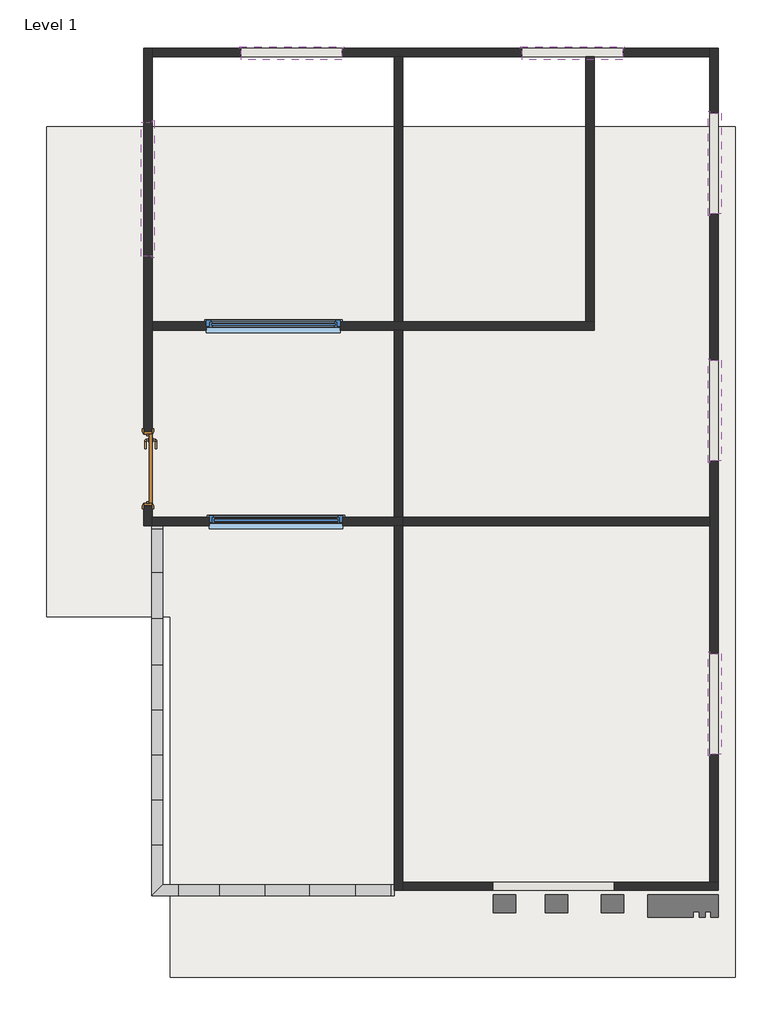
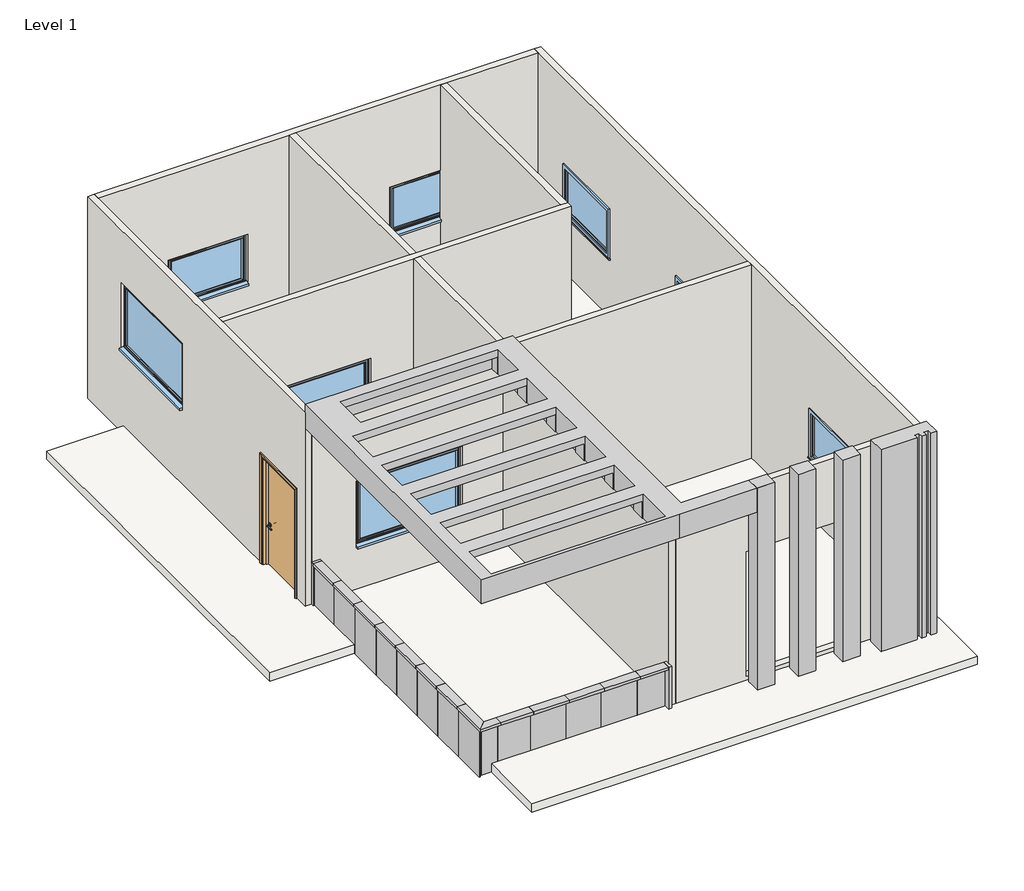
# One storey, incomplete: 16 members, 14 plates, 11 walls, 8 windows, 1 door, 1 proxy, 1 roof.
"""IFC4 building model written with IfcOpenShell, lengths in millimetres."""

from ifc_helpers import new_model, si_unit, frame, origin, place, context, project, spatial, polyline, outline, extrude, faceted_brep, transform, mapped, element, save
from components import generic_models_2_generic_models_2_13626f08, doors_intsgl_1010x2110mm_a785dbed, rectangular_mullion_50x150mm_cc836158, rectangular_mullion_50x150mm_b9b5507c, rectangular_mullion_50x150mm_11f8c00f, rectangular_mullion_50x150mm_61ade493, rectangular_mullion_50x150mm_d3e7ce4f, rectangular_mullion_50x150mm_3c996cd3, rectangular_mullion_50x150mm_ded1ff81, rectangular_mullion_50x150mm_6d544d31, system_panel_glazed_ffea3bad, system_panel_glazed_b26c39eb, system_panel_glazed_8bec2438, system_panel_glazed_703d63a0, system_panel_glazed_36803b61, system_panel_glazed_d3aa7d51, windows_sgl_plain_1360x910mm_1fca1195, windows_sgl_plain_1810x1210mm_100c968f

model = new_model("IFC4")

# Units and contexts
model_context = context("Model", 3, world=origin())
ifc_project = project(units=[si_unit("LENGTHUNIT", "METRE", prefix="MILLI")], contexts=[model_context])

# Site, building, storey
site = spatial("IfcSite", under=ifc_project)
building = spatial("IfcBuilding", under=site)
storey = spatial("IfcBuildingStorey", under=building, Name="Level 1", Elevation=3048.0)

# Proxy
placement = place(None, origin())
generic_models_2_generic_models_2_shape = generic_models_2_generic_models_2_13626f08(model_context)
element("IfcBuildingElementProxy", 1, Name="Generic Models 2 : Generic Models 2", ObjectType="Generic Models 2 : Generic Models 2", at=placement, inside=storey, context=model_context, shape_type="MappedRepresentation", body=[
    mapped(generic_models_2_generic_models_2_shape, transform((0.0, 0.0, 0.0), x_axis=(1.0, 0.0, 0.0), y_axis=(0.0, 1.0, 0.0), z_axis=(0.0, 0.0, 1.0))),
])

# Door
doors_intsgl_1010x2110mm_shape = doors_intsgl_1010x2110mm_a785dbed(model_context)
element("IfcDoor", 2, ObjectType="Doors_IntSgl : 1010x2110mm", at=placement, inside=storey, context=model_context, shape_type="MappedRepresentation", body=[
    mapped(doors_intsgl_1010x2110mm_shape, transform((-7880.7025595, 2466.5132107, 3048.0), x_axis=(0.0, -1.0, 0.0), y_axis=(1.0, 0.0, 0.0), z_axis=(0.0, 0.0, 1.0))),
])

# Members
rectangular_mullion_50x150mm_shape = rectangular_mullion_50x150mm_cc836158(model_context)
element("IfcMember", 3, ObjectType="Rectangular Mullion : 50x150mm", at=placement, inside=storey, context=model_context, shape_type="MappedRepresentation", body=[
    mapped(rectangular_mullion_50x150mm_shape, transform((-7753.7025595, 1694.8132107, 3048.0), x_axis=(0.0, 1.0, 0.0), y_axis=(1.0, 0.0, 0.0), z_axis=(0.0, 0.0, -1.0))),
])
element("IfcMember", 4, ObjectType="Rectangular Mullion : 50x150mm", at=placement, inside=storey, context=model_context, shape_type="MappedRepresentation", body=[
    mapped(rectangular_mullion_50x150mm_shape, transform((-4546.9525595, -3239.1367893, 3048.0), x_axis=(1.0, 0.0, 0.0), y_axis=(0.0, -1.0, 0.0), z_axis=(0.0, 0.0, -1.0))),
])
rectangular_mullion_50x150mm_2_shape = rectangular_mullion_50x150mm_b9b5507c(model_context)
element("IfcMember", 5, ObjectType="Rectangular Mullion : 50x150mm", at=placement, inside=storey, context=model_context, shape_type="MappedRepresentation", body=[
    mapped(rectangular_mullion_50x150mm_2_shape, transform((-4596.9525595, -3239.1367893, 3962.4), x_axis=(0.0, 0.0, 1.0), y_axis=(0.0, -1.0, 0.0), z_axis=(1.0, 0.0, 0.0))),
])
rectangular_mullion_50x150mm_3_shape = rectangular_mullion_50x150mm_11f8c00f(model_context)
element("IfcMember", 6, ObjectType="Rectangular Mullion : 50x150mm", at=placement, inside=storey, context=model_context, shape_type="MappedRepresentation", body=[
    mapped(rectangular_mullion_50x150mm_3_shape, transform((-5080.3525595, -3239.1367893, 3962.4), x_axis=(0.0, 0.0, 1.0), y_axis=(0.0, -1.0, 0.0), z_axis=(1.0, 0.0, 0.0))),
])
element("IfcMember", 7, ObjectType="Rectangular Mullion : 50x150mm", at=placement, inside=storey, context=model_context, shape_type="MappedRepresentation", body=[
    mapped(rectangular_mullion_50x150mm_3_shape, transform((-5689.9525595, -3239.1367893, 3962.4), x_axis=(0.0, 0.0, 1.0), y_axis=(0.0, -1.0, 0.0), z_axis=(1.0, 0.0, 0.0))),
])
element("IfcMember", 8, ObjectType="Rectangular Mullion : 50x150mm", at=placement, inside=storey, context=model_context, shape_type="MappedRepresentation", body=[
    mapped(rectangular_mullion_50x150mm_3_shape, transform((-6299.5525595, -3239.1367893, 3962.4), x_axis=(0.0, 0.0, 1.0), y_axis=(0.0, -1.0, 0.0), z_axis=(1.0, 0.0, 0.0))),
])
element("IfcMember", 9, ObjectType="Rectangular Mullion : 50x150mm", at=placement, inside=storey, context=model_context, shape_type="MappedRepresentation", body=[
    mapped(rectangular_mullion_50x150mm_3_shape, transform((-7753.7025595, -2019.9367893, 3962.4), x_axis=(0.0, 0.0, 1.0), y_axis=(1.0, 0.0, 0.0), z_axis=(0.0, 1.0, 0.0))),
])
element("IfcMember", 10, ObjectType="Rectangular Mullion : 50x150mm", at=placement, inside=storey, context=model_context, shape_type="MappedRepresentation", body=[
    mapped(rectangular_mullion_50x150mm_3_shape, transform((-7753.7025595, -1410.3367893, 3962.4), x_axis=(0.0, 0.0, 1.0), y_axis=(1.0, 0.0, 0.0), z_axis=(0.0, 1.0, 0.0))),
])
element("IfcMember", 11, ObjectType="Rectangular Mullion : 50x150mm", at=placement, inside=storey, context=model_context, shape_type="MappedRepresentation", body=[
    mapped(rectangular_mullion_50x150mm_3_shape, transform((-7753.7025595, -800.7367893, 3962.4), x_axis=(0.0, 0.0, 1.0), y_axis=(1.0, 0.0, 0.0), z_axis=(0.0, 1.0, 0.0))),
])
element("IfcMember", 12, ObjectType="Rectangular Mullion : 50x150mm", at=placement, inside=storey, context=model_context, shape_type="MappedRepresentation", body=[
    mapped(rectangular_mullion_50x150mm_3_shape, transform((-7753.7025595, -191.1367893, 3962.4), x_axis=(0.0, 0.0, 1.0), y_axis=(1.0, 0.0, 0.0), z_axis=(0.0, 1.0, 0.0))),
])
rectangular_mullion_50x150mm_4_shape = rectangular_mullion_50x150mm_61ade493(model_context)
element("IfcMember", 13, ObjectType="Rectangular Mullion : 50x150mm", at=placement, inside=storey, context=model_context, shape_type="MappedRepresentation", body=[
    mapped(rectangular_mullion_50x150mm_4_shape, transform((-6909.1525595, -3239.1367893, 3962.4), x_axis=(0.0, 0.0, 1.0), y_axis=(0.0, -1.0, 0.0), z_axis=(1.0, 0.0, 0.0))),
])
rectangular_mullion_50x150mm_5_shape = rectangular_mullion_50x150mm_d3e7ce4f(model_context)
element("IfcMember", 14, ObjectType="Rectangular Mullion : 50x150mm", at=placement, inside=storey, context=model_context, shape_type="MappedRepresentation", body=[
    mapped(rectangular_mullion_50x150mm_5_shape, transform((-7753.7025595, -2629.5367893, 3962.4), x_axis=(0.0, 0.0, 1.0), y_axis=(1.0, 0.0, 0.0), z_axis=(0.0, 1.0, 0.0))),
])
rectangular_mullion_50x150mm_6_shape = rectangular_mullion_50x150mm_3c996cd3(model_context)
element("IfcMember", 15, ObjectType="Rectangular Mullion : 50x150mm", at=placement, inside=storey, context=model_context, shape_type="MappedRepresentation", body=[
    mapped(rectangular_mullion_50x150mm_6_shape, transform((-7472.1858928, -3239.1367893, 3962.4), x_axis=(0.0, 0.0, 1.0), y_axis=(0.0, -1.0, 0.0), z_axis=(1.0, 0.0, 0.0))),
])
rectangular_mullion_50x150mm_7_shape = rectangular_mullion_50x150mm_ded1ff81(model_context)
element("IfcMember", 16, ObjectType="Rectangular Mullion : 50x150mm", at=placement, inside=storey, context=model_context, shape_type="MappedRepresentation", body=[
    mapped(rectangular_mullion_50x150mm_7_shape, transform((-7753.7025595, 437.5132107, 3962.4), x_axis=(0.0, 0.0, 1.0), y_axis=(1.0, 0.0, 0.0), z_axis=(0.0, 1.0, 0.0))),
])
element("IfcMember", 17, ObjectType="Rectangular Mullion : 50x150mm", at=placement, inside=storey, context=model_context, shape_type="MappedRepresentation", body=[
    mapped(rectangular_mullion_50x150mm_7_shape, transform((-7753.7025595, 1066.1632107, 3962.4), x_axis=(0.0, 0.0, 1.0), y_axis=(1.0, 0.0, 0.0), z_axis=(0.0, 1.0, 0.0))),
])
rectangular_mullion_50x150mm_8_shape = rectangular_mullion_50x150mm_6d544d31(model_context)
element("IfcMember", 18, ObjectType="Rectangular Mullion : 50x150mm", at=placement, inside=storey, context=model_context, shape_type="MappedRepresentation", body=[
    mapped(rectangular_mullion_50x150mm_8_shape, transform((-7753.7025595, 1644.8132107, 3962.4), x_axis=(0.0, 0.0, 1.0), y_axis=(1.0, 0.0, 0.0), z_axis=(0.0, 1.0, 0.0))),
])

# Plates
system_panel_glazed_shape = system_panel_glazed_ffea3bad(model_context)
element("IfcPlate", 19, ObjectType="System Panel : Glazed", at=placement, inside=storey, context=model_context, shape_type="MappedRepresentation", body=[
    mapped(system_panel_glazed_shape, transform((-4838.6525595, -3239.1367893, 3048.0), x_axis=(1.0, 0.0, 0.0), y_axis=(0.0, 1.0, 0.0), z_axis=(0.0, 0.0, 1.0))),
])
system_panel_glazed_2_shape = system_panel_glazed_b26c39eb(model_context)
element("IfcPlate", 20, ObjectType="System Panel : Glazed", at=placement, inside=storey, context=model_context, shape_type="MappedRepresentation", body=[
    mapped(system_panel_glazed_2_shape, transform((-7753.7025595, -2934.3367893, 3048.0), x_axis=(0.0, 1.0, 0.0), y_axis=(-1.0, 0.0, 0.0), z_axis=(0.0, 0.0, 1.0))),
])
element("IfcPlate", 21, ObjectType="System Panel : Glazed", at=placement, inside=storey, context=model_context, shape_type="MappedRepresentation", body=[
    mapped(system_panel_glazed_2_shape, transform((-5385.1525595, -3239.1367893, 3048.0), x_axis=(1.0, 0.0, 0.0), y_axis=(0.0, 1.0, 0.0), z_axis=(0.0, 0.0, 1.0))),
])
element("IfcPlate", 22, ObjectType="System Panel : Glazed", at=placement, inside=storey, context=model_context, shape_type="MappedRepresentation", body=[
    mapped(system_panel_glazed_2_shape, transform((-5994.7525595, -3239.1367893, 3048.0), x_axis=(1.0, 0.0, 0.0), y_axis=(0.0, 1.0, 0.0), z_axis=(0.0, 0.0, 1.0))),
])
element("IfcPlate", 23, ObjectType="System Panel : Glazed", at=placement, inside=storey, context=model_context, shape_type="MappedRepresentation", body=[
    mapped(system_panel_glazed_2_shape, transform((-6604.3525595, -3239.1367893, 3048.0), x_axis=(1.0, 0.0, 0.0), y_axis=(0.0, 1.0, 0.0), z_axis=(0.0, 0.0, 1.0))),
])
element("IfcPlate", 24, ObjectType="System Panel : Glazed", at=placement, inside=storey, context=model_context, shape_type="MappedRepresentation", body=[
    mapped(system_panel_glazed_2_shape, transform((-7753.7025595, -2324.7367893, 3048.0), x_axis=(0.0, 1.0, 0.0), y_axis=(-1.0, 0.0, 0.0), z_axis=(0.0, 0.0, 1.0))),
])
element("IfcPlate", 25, ObjectType="System Panel : Glazed", at=placement, inside=storey, context=model_context, shape_type="MappedRepresentation", body=[
    mapped(system_panel_glazed_2_shape, transform((-7753.7025595, -1715.1367893, 3048.0), x_axis=(0.0, 1.0, 0.0), y_axis=(-1.0, 0.0, 0.0), z_axis=(0.0, 0.0, 1.0))),
])
element("IfcPlate", 26, ObjectType="System Panel : Glazed", at=placement, inside=storey, context=model_context, shape_type="MappedRepresentation", body=[
    mapped(system_panel_glazed_2_shape, transform((-7753.7025595, -1105.5367893, 3048.0), x_axis=(0.0, 1.0, 0.0), y_axis=(-1.0, 0.0, 0.0), z_axis=(0.0, 0.0, 1.0))),
])
element("IfcPlate", 27, ObjectType="System Panel : Glazed", at=placement, inside=storey, context=model_context, shape_type="MappedRepresentation", body=[
    mapped(system_panel_glazed_2_shape, transform((-7753.7025595, -495.9367893, 3048.0), x_axis=(0.0, 1.0, 0.0), y_axis=(-1.0, 0.0, 0.0), z_axis=(0.0, 0.0, 1.0))),
])
system_panel_glazed_3_shape = system_panel_glazed_8bec2438(model_context)
element("IfcPlate", 28, ObjectType="System Panel : Glazed", at=placement, inside=storey, context=model_context, shape_type="MappedRepresentation", body=[
    mapped(system_panel_glazed_3_shape, transform((-7190.6692261, -3239.1367893, 3048.0), x_axis=(1.0, 0.0, 0.0), y_axis=(0.0, 1.0, 0.0), z_axis=(0.0, 0.0, 1.0))),
])
system_panel_glazed_4_shape = system_panel_glazed_703d63a0(model_context)
element("IfcPlate", 29, ObjectType="System Panel : Glazed", at=placement, inside=storey, context=model_context, shape_type="MappedRepresentation", body=[
    mapped(system_panel_glazed_4_shape, transform((-7612.9442261, -3239.1367893, 3048.0), x_axis=(1.0, 0.0, 0.0), y_axis=(0.0, 1.0, 0.0), z_axis=(0.0, 0.0, 1.0))),
])
system_panel_glazed_5_shape = system_panel_glazed_36803b61(model_context)
element("IfcPlate", 30, ObjectType="System Panel : Glazed", at=placement, inside=storey, context=model_context, shape_type="MappedRepresentation", body=[
    mapped(system_panel_glazed_5_shape, transform((-7753.7025595, 123.1882107, 3048.0), x_axis=(0.0, 1.0, 0.0), y_axis=(-1.0, 0.0, 0.0), z_axis=(0.0, 0.0, 1.0))),
])
element("IfcPlate", 31, ObjectType="System Panel : Glazed", at=placement, inside=storey, context=model_context, shape_type="MappedRepresentation", body=[
    mapped(system_panel_glazed_5_shape, transform((-7753.7025595, 751.8382107, 3048.0), x_axis=(0.0, 1.0, 0.0), y_axis=(-1.0, 0.0, 0.0), z_axis=(0.0, 0.0, 1.0))),
])
system_panel_glazed_6_shape = system_panel_glazed_d3aa7d51(model_context)
element("IfcPlate", 32, ObjectType="System Panel : Glazed", at=placement, inside=storey, context=model_context, shape_type="MappedRepresentation", body=[
    mapped(system_panel_glazed_6_shape, transform((-7753.7025595, 1355.4882107, 3048.0), x_axis=(0.0, 1.0, 0.0), y_axis=(-1.0, 0.0, 0.0), z_axis=(0.0, 0.0, 1.0))),
])

# Roof
element("IfcRoof", 33, ObjectType="6\"", at=placement, inside=storey, context=model_context, shape_type="SweptSolid", body=[
    extrude(outline(polyline([(-9253.7144009, 7090.2001437), (61.7355991, 7090.2001437), (61.7355991, -4415.9998563), (-7577.3144009, -4415.9998563), (-7577.3144009, 460.8001437), (-9253.7144009, 460.8001437), (-9253.7144009, 7090.2001437)])), frame((0.0, 0.0, 3048.0), z_axis=(0.0, 0.0, 1.0), x_axis=(1.0, 0.0, 0.0)), (0.0, 0.0, 1.0), 152.4),
])

# Walls
element("IfcWall", 34, ObjectType="4.5\" wall", at=placement, inside=storey, context=model_context, shape_type="Brep", body=[
    faceted_brep([(-7823.5525595, 8152.7632107, 6705.6), (-7823.5525595, 8038.4632107, 6705.6), (-7823.5525595, 4457.0632107, 6705.6), (-7823.5525595, 4342.7632107, 6705.6), (-7823.5525595, 1809.1132107, 6705.6), (-7823.5525595, 1694.8132107, 6705.6), (-7823.5525595, 1694.8132107, 3048.0), (-7823.5525595, 1809.1132107, 3048.0), (-7823.5525595, 1961.5132107, 3048.0), (-7823.5525595, 1961.5132107, 5158.0), (-7823.5525595, 2971.5132107, 5158.0), (-7823.5525595, 2971.5132107, 3048.0), (-7823.5525595, 4342.7632107, 3048.0), (-7823.5525595, 4457.0632107, 3048.0), (-7823.5525595, 8038.4632107, 3048.0), (-7823.5525595, 8152.7632107, 3048.0), (-7823.5525595, 5342.7632107, 4542.5182366), (-7823.5525595, 5342.7632107, 5752.5182366), (-7823.5525595, 7152.7632107, 5752.5182366), (-7823.5525595, 7152.7632107, 4542.5182366), (-7937.8525595, 1694.8132107, 6705.6), (-7937.8525595, 8152.7632107, 6705.6), (-7937.8525595, 8152.7632107, 3048.0), (-7937.8525595, 2971.5132107, 3048.0), (-7937.8525595, 2971.5132107, 5158.0), (-7937.8525595, 1961.5132107, 5158.0), (-7937.8525595, 1961.5132107, 3048.0), (-7937.8525595, 1694.8132107, 3048.0), (-7937.8525595, 5342.7632107, 5752.5182366), (-7937.8525595, 5342.7632107, 4542.5182366), (-7937.8525595, 7152.7632107, 4542.5182366), (-7937.8525595, 7152.7632107, 5752.5182366)], [[[0, 1, 2, 3, 4, 5, 6, 7, 8, 9, 10, 11, 12, 13, 14, 15], [16, 17, 18, 19]], [[20, 21, 22, 23, 24, 25, 26, 27], [28, 29, 30, 31]], [[6, 27, 26, 8, 7]], [[22, 15, 14, 13, 12, 11, 23]], [[5, 4, 3, 2, 1, 0, 21, 20]], [[6, 5, 20, 27]], [[0, 15, 22, 21]], [[29, 28, 17, 16]], [[30, 29, 16, 19]], [[31, 30, 19, 18]], [[28, 31, 18, 17]], [[25, 9, 8, 26]], [[9, 25, 24, 10]], [[10, 24, 23, 11]]]),
])
element("IfcWall", 35, ObjectType="4.5\" wall", at=placement, inside=storey, context=model_context, shape_type="Brep", body=[
    faceted_brep([(-7823.5525595, 1694.8132107, 3048.0), (-4546.9525595, 1694.8132107, 3048.0), (-4432.6525595, 1694.8132107, 3048.0), (-4432.6525595, 1694.8132107, 6705.6), (-4546.9525595, 1694.8132107, 6705.6), (-7823.5525595, 1694.8132107, 6705.6), (-5245.3275595, 1694.8132107, 5158.0), (-5245.3275595, 1694.8132107, 3948.0), (-7055.3275595, 1694.8132107, 3948.0), (-7055.3275595, 1694.8132107, 5158.0), (-7823.5525595, 1809.1132107, 3048.0), (-7823.5525595, 1809.1132107, 6705.6), (-4546.9525595, 1809.1132107, 6705.6), (-4432.6525595, 1809.1132107, 6705.6), (-4432.6525595, 1809.1132107, 3048.0), (-4546.9525595, 1809.1132107, 3048.0), (-5245.3275595, 1809.1132107, 5158.0), (-7055.3275595, 1809.1132107, 5158.0), (-7055.3275595, 1809.1132107, 3948.0), (-5245.3275595, 1809.1132107, 3948.0)], [[[0, 1, 2, 3, 4, 5], [6, 7, 8, 9]], [[10, 11, 12, 13, 14, 15], [16, 17, 18, 19]], [[2, 1, 0, 10, 15, 14]], [[5, 4, 3, 13, 12, 11]], [[0, 5, 11, 10]], [[3, 2, 14, 13]], [[7, 6, 16, 19]], [[8, 7, 19, 18]], [[9, 8, 18, 17]], [[6, 9, 17, 16]]]),
])
element("IfcWall", 36, ObjectType="4.5\" wall", at=placement, inside=storey, context=model_context, shape_type="Brep", body=[
    faceted_brep([(-4546.9525595, 1694.8132107, 3048.0), (-4546.9525595, -3239.1367893, 3048.0), (-4546.9525595, -3239.1367893, 6705.6), (-4546.9525595, 1694.8132107, 6705.6), (-4432.6525595, 1694.8132107, 3048.0), (-4432.6525595, 1694.8132107, 6705.6), (-4432.6525595, -3124.8367893, 6705.6), (-4432.6525595, -3239.1367893, 6705.6), (-4432.6525595, -3239.1367893, 3048.0), (-4432.6525595, -3124.8367893, 3048.0)], [[[0, 1, 2, 3]], [[4, 5, 6, 7, 8, 9]], [[1, 0, 4, 9, 8]], [[3, 2, 7, 6, 5]], [[0, 3, 5, 4]], [[2, 1, 8, 7]]]),
])
element("IfcWall", 37, ObjectType="4.5\" wall", at=placement, inside=storey, context=model_context, shape_type="Brep", body=[
    faceted_brep([(-4432.6525595, -3239.1367893, 3048.0), (-165.4525595, -3239.1367893, 3048.0), (-165.4525595, -3239.1367893, 6705.6), (-4432.6525595, -3239.1367893, 6705.6), (-1572.6025595, -3239.1367893, 3273.0), (-3219.8025595, -3239.1367893, 3273.0), (-3219.8025595, -3239.1367893, 5523.0), (-1572.6025595, -3239.1367893, 5523.0), (-4432.6525595, -3124.8367893, 3048.0), (-4432.6525595, -3124.8367893, 6705.6), (-279.7525595, -3124.8367893, 6705.6), (-165.4525595, -3124.8367893, 6705.6), (-165.4525595, -3124.8367893, 3048.0), (-279.7525595, -3124.8367893, 3048.0), (-1572.6025595, -3124.8367893, 3273.0), (-1572.6025595, -3124.8367893, 5523.0), (-3219.8025595, -3124.8367893, 5523.0), (-3219.8025595, -3124.8367893, 3273.0)], [[[0, 1, 2, 3], [4, 5, 6, 7]], [[8, 9, 10, 11, 12, 13], [14, 15, 16, 17]], [[0, 3, 9, 8]], [[2, 1, 12, 11]], [[1, 0, 8, 13, 12]], [[3, 2, 11, 10, 9]], [[5, 4, 14, 17]], [[6, 5, 17, 16]], [[7, 6, 16, 15]], [[4, 7, 15, 14]]]),
])
element("IfcWall", 38, ObjectType="4.5\" wall", at=placement, inside=storey, context=model_context, shape_type="Brep", body=[
    faceted_brep([(-165.4525595, -3124.8367893, 3048.0), (-165.4525595, 8152.7632107, 3048.0), (-165.4525595, 8152.7632107, 6705.6), (-165.4525595, -3124.8367893, 6705.6), (-165.4525595, 7276.4632107, 5158.0), (-165.4525595, 7276.4632107, 4248.0), (-165.4525595, 5916.4632107, 4248.0), (-165.4525595, 5916.4632107, 5158.0), (-165.4525595, 3931.1132107, 5158.0), (-165.4525595, 3931.1132107, 4248.0), (-165.4525595, 2571.1132107, 4248.0), (-165.4525595, 2571.1132107, 5158.0), (-165.4525595, -35.0117893, 5158.0), (-165.4525595, -35.0117893, 4248.0), (-165.4525595, -1395.0117893, 4248.0), (-165.4525595, -1395.0117893, 5158.0), (-279.7525595, -3124.8367893, 3048.0), (-279.7525595, -3124.8367893, 6705.6), (-279.7525595, 1694.8132107, 6705.6), (-279.7525595, 1809.1132107, 6705.6), (-279.7525595, 8038.4632107, 6705.6), (-279.7525595, 8152.7632107, 6705.6), (-279.7525595, 8152.7632107, 3048.0), (-279.7525595, 8038.4632107, 3048.0), (-279.7525595, 1809.1132107, 3048.0), (-279.7525595, 1694.8132107, 3048.0), (-279.7525595, 7276.4632107, 5158.0), (-279.7525595, 5916.4632107, 5158.0), (-279.7525595, 5916.4632107, 4248.0), (-279.7525595, 7276.4632107, 4248.0), (-279.7525595, 3931.1132107, 5158.0), (-279.7525595, 2571.1132107, 5158.0), (-279.7525595, 2571.1132107, 4248.0), (-279.7525595, 3931.1132107, 4248.0), (-279.7525595, -35.0117893, 5158.0), (-279.7525595, -1395.0117893, 5158.0), (-279.7525595, -1395.0117893, 4248.0), (-279.7525595, -35.0117893, 4248.0)], [[[0, 1, 2, 3], [4, 5, 6, 7], [8, 9, 10, 11], [12, 13, 14, 15]], [[16, 17, 18, 19, 20, 21, 22, 23, 24, 25], [26, 27, 28, 29], [30, 31, 32, 33], [34, 35, 36, 37]], [[1, 0, 16, 25, 24, 23, 22]], [[3, 2, 21, 20, 19, 18, 17]], [[0, 3, 17, 16]], [[2, 1, 22, 21]], [[5, 4, 26, 29]], [[6, 5, 29, 28]], [[7, 6, 28, 27]], [[4, 7, 27, 26]], [[9, 8, 30, 33]], [[10, 9, 33, 32]], [[11, 10, 32, 31]], [[8, 11, 31, 30]], [[13, 12, 34, 37]], [[14, 13, 37, 36]], [[15, 14, 36, 35]], [[12, 15, 35, 34]]]),
])
element("IfcWall", 39, ObjectType="4.5\" wall", at=placement, inside=storey, context=model_context, shape_type="Brep", body=[
    faceted_brep([(-279.7525595, 8152.7632107, 3048.0), (-7823.5525595, 8152.7632107, 3048.0), (-7823.5525595, 8152.7632107, 6705.6), (-279.7525595, 8152.7632107, 6705.6), (-1460.8525595, 8152.7632107, 4248.0), (-1460.8525595, 8152.7632107, 5158.0), (-2820.8525595, 8152.7632107, 5158.0), (-2820.8525595, 8152.7632107, 4248.0), (-5259.2525595, 8152.7632107, 4248.0), (-5259.2525595, 8152.7632107, 5158.0), (-6619.2525595, 8152.7632107, 5158.0), (-6619.2525595, 8152.7632107, 4248.0), (-7823.5525595, 8038.4632107, 3048.0), (-4546.9525595, 8038.4632107, 3048.0), (-4432.6525595, 8038.4632107, 3048.0), (-1956.1525595, 8038.4632107, 3048.0), (-1841.8525595, 8038.4632107, 3048.0), (-279.7525595, 8038.4632107, 3048.0), (-279.7525595, 8038.4632107, 6705.6), (-1841.8525595, 8038.4632107, 6705.6), (-1956.1525595, 8038.4632107, 6705.6), (-4432.6525595, 8038.4632107, 6705.6), (-4546.9525595, 8038.4632107, 6705.6), (-7823.5525595, 8038.4632107, 6705.6), (-1460.8525595, 8038.4632107, 5158.0), (-1460.8525595, 8038.4632107, 4248.0), (-2820.8525595, 8038.4632107, 4248.0), (-2820.8525595, 8038.4632107, 5158.0), (-5259.2525595, 8038.4632107, 5158.0), (-5259.2525595, 8038.4632107, 4248.0), (-6619.2525595, 8038.4632107, 4248.0), (-6619.2525595, 8038.4632107, 5158.0)], [[[0, 1, 2, 3], [4, 5, 6, 7], [8, 9, 10, 11]], [[12, 13, 14, 15, 16, 17, 18, 19, 20, 21, 22, 23], [24, 25, 26, 27], [28, 29, 30, 31]], [[1, 0, 17, 16, 15, 14, 13, 12]], [[3, 2, 23, 22, 21, 20, 19, 18]], [[0, 3, 18, 17]], [[2, 1, 12, 23]], [[24, 5, 4, 25]], [[25, 4, 7, 26]], [[26, 7, 6, 27]], [[5, 24, 27, 6]], [[28, 9, 8, 29]], [[29, 8, 11, 30]], [[30, 11, 10, 31]], [[9, 28, 31, 10]]]),
])
element("IfcWall", 40, ObjectType="4.5\" wall", at=placement, inside=storey, context=model_context, shape_type="Brep", body=[
    faceted_brep([(-7823.5525595, 4342.7632107, 3048.0), (-4546.9525595, 4342.7632107, 3048.0), (-4432.6525595, 4342.7632107, 3048.0), (-1841.8525595, 4342.7632107, 3048.0), (-1841.8525595, 4342.7632107, 6705.6), (-4432.6525595, 4342.7632107, 6705.6), (-4546.9525595, 4342.7632107, 6705.6), (-7823.5525595, 4342.7632107, 6705.6), (-5280.2525595, 4342.7632107, 5158.0), (-5280.2525595, 4342.7632107, 3948.0), (-7090.2525595, 4342.7632107, 3948.0), (-7090.2525595, 4342.7632107, 5158.0), (-1841.8525595, 4457.0632107, 3048.0), (-1956.1525595, 4457.0632107, 3048.0), (-4432.6525595, 4457.0632107, 3048.0), (-4546.9525595, 4457.0632107, 3048.0), (-7823.5525595, 4457.0632107, 3048.0), (-7823.5525595, 4457.0632107, 6705.6), (-4546.9525595, 4457.0632107, 6705.6), (-4432.6525595, 4457.0632107, 6705.6), (-1956.1525595, 4457.0632107, 6705.6), (-1841.8525595, 4457.0632107, 6705.6), (-5280.2525595, 4457.0632107, 3948.0), (-5280.2525595, 4457.0632107, 5158.0), (-7090.2525595, 4457.0632107, 5158.0), (-7090.2525595, 4457.0632107, 3948.0)], [[[0, 1, 2, 3, 4, 5, 6, 7], [8, 9, 10, 11]], [[12, 13, 14, 15, 16, 17, 18, 19, 20, 21], [22, 23, 24, 25]], [[3, 2, 1, 0, 16, 15, 14, 13, 12]], [[7, 6, 5, 4, 21, 20, 19, 18, 17]], [[0, 7, 17, 16]], [[4, 3, 12, 21]], [[8, 23, 22, 9]], [[9, 22, 25, 10]], [[10, 25, 24, 11]], [[23, 8, 11, 24]]]),
])
element("IfcWall", 41, ObjectType="4.5\" wall", at=placement, inside=storey, context=model_context, shape_type="SweptSolid", body=[
    extrude(outline(polyline([(-4546.9525595, 1809.1132107), (-4546.9525595, 4342.7632107), (-4432.6525595, 4342.7632107), (-4432.6525595, 1809.1132107), (-4546.9525595, 1809.1132107)])), frame((0.0, 0.0, 3048.0), z_axis=(0.0, 0.0, 1.0), x_axis=(1.0, 0.0, 0.0)), (0.0, 0.0, 1.0), 3657.6),
])
element("IfcWall", 42, ObjectType="4.5\" wall", at=placement, inside=storey, context=model_context, shape_type="SweptSolid", body=[
    extrude(outline(polyline([(-1841.8525595, 8038.4632107), (-1841.8525595, 4457.0632107), (-1956.1525595, 4457.0632107), (-1956.1525595, 8038.4632107), (-1841.8525595, 8038.4632107)])), frame((0.0, 0.0, 3048.0), z_axis=(0.0, 0.0, 1.0), x_axis=(1.0, 0.0, 0.0)), (0.0, 0.0, 1.0), 3657.6),
])
element("IfcWall", 43, ObjectType="4.5\" wall", at=placement, inside=storey, context=model_context, shape_type="SweptSolid", body=[
    extrude(outline(polyline([(-4432.6525595, 8038.4632107), (-4432.6525595, 4457.0632107), (-4546.9525595, 4457.0632107), (-4546.9525595, 8038.4632107), (-4432.6525595, 8038.4632107)])), frame((0.0, 0.0, 3048.0), z_axis=(0.0, 0.0, 1.0), x_axis=(1.0, 0.0, 0.0)), (0.0, 0.0, 1.0), 3657.6),
])
element("IfcWall", 44, ObjectType="4.5\" wall", at=placement, inside=storey, context=model_context, shape_type="SweptSolid", body=[
    extrude(outline(polyline([(-279.7525595, 1694.8132107), (-4432.6525595, 1694.8132107), (-4432.6525595, 1809.1132107), (-279.7525595, 1809.1132107), (-279.7525595, 1694.8132107)])), frame((0.0, 0.0, 3048.0), z_axis=(0.0, 0.0, 1.0), x_axis=(1.0, 0.0, 0.0)), (0.0, 0.0, 1.0), 3657.6),
])

# Windows
windows_sgl_plain_1360x910mm_shape = windows_sgl_plain_1360x910mm_1fca1195(model_context)
element("IfcWindow", 45, ObjectType="Windows_Sgl_Plain : 1360x910mm", at=placement, inside=storey, context=model_context, shape_type="MappedRepresentation", body=[
    mapped(windows_sgl_plain_1360x910mm_shape, transform((-231.0591273, 6596.4632107, 3048.0), x_axis=(0.0, -1.0, 0.0), y_axis=(1.0, 0.0, 0.0), z_axis=(0.0, 0.0, 1.0))),
])
element("IfcWindow", 46, ObjectType="Windows_Sgl_Plain : 1360x910mm", at=placement, inside=storey, context=model_context, shape_type="MappedRepresentation", body=[
    mapped(windows_sgl_plain_1360x910mm_shape, transform((-231.0591273, 3251.1132107, 3048.0), x_axis=(0.0, -1.0, 0.0), y_axis=(1.0, 0.0, 0.0), z_axis=(0.0, 0.0, 1.0))),
])
element("IfcWindow", 47, ObjectType="Windows_Sgl_Plain : 1360x910mm", at=placement, inside=storey, context=model_context, shape_type="MappedRepresentation", body=[
    mapped(windows_sgl_plain_1360x910mm_shape, transform((-231.0591273, -715.0117893, 3048.0), x_axis=(0.0, -1.0, 0.0), y_axis=(1.0, 0.0, 0.0), z_axis=(0.0, 0.0, 1.0))),
])
element("IfcWindow", 48, ObjectType="Windows_Sgl_Plain : 1360x910mm", at=placement, inside=storey, context=model_context, shape_type="MappedRepresentation", body=[
    mapped(windows_sgl_plain_1360x910mm_shape, transform((-2140.8525595, 8104.0697785, 3048.0), x_axis=(-1.0, 0.0, 0.0), y_axis=(0.0, -1.0, 0.0), z_axis=(0.0, 0.0, 1.0))),
])
element("IfcWindow", 49, ObjectType="Windows_Sgl_Plain : 1360x910mm", at=placement, inside=storey, context=model_context, shape_type="MappedRepresentation", body=[
    mapped(windows_sgl_plain_1360x910mm_shape, transform((-5939.2525595, 8104.0697785, 3048.0), x_axis=(-1.0, 0.0, 0.0), y_axis=(0.0, -1.0, 0.0), z_axis=(0.0, 0.0, 1.0))),
])
windows_sgl_plain_1810x1210mm_shape = windows_sgl_plain_1810x1210mm_100c968f(model_context)
element("IfcWindow", 50, ObjectType="Windows_Sgl_Plain : 1810x1210mm", at=placement, inside=storey, context=model_context, shape_type="MappedRepresentation", body=[
    mapped(windows_sgl_plain_1810x1210mm_shape, transform((-6150.3275595, 1760.4197785, 3048.0), x_axis=(-1.0, 0.0, 0.0), y_axis=(0.0, -1.0, 0.0), z_axis=(0.0, 0.0, 1.0))),
])
element("IfcWindow", 51, ObjectType="Windows_Sgl_Plain : 1810x1210mm", at=placement, inside=storey, context=model_context, shape_type="MappedRepresentation", body=[
    mapped(windows_sgl_plain_1810x1210mm_shape, transform((-6185.2525595, 4408.3697785, 3048.0), x_axis=(-1.0, 0.0, 0.0), y_axis=(0.0, -1.0, 0.0), z_axis=(0.0, 0.0, 1.0))),
])
element("IfcWindow", 52, ObjectType="Windows_Sgl_Plain : 1810x1210mm", at=placement, inside=storey, context=model_context, shape_type="MappedRepresentation", body=[
    mapped(windows_sgl_plain_1810x1210mm_shape, transform((-7872.2459916, 6247.7632107, 3642.5182366), x_axis=(0.0, 1.0, 0.0), y_axis=(-1.0, 0.0, 0.0), z_axis=(0.0, 0.0, 1.0))),
])

save(model, "model.ifc")

# Revit data of these elements
# Type "Doors_IntSgl : 1010x2110mm"
#   Construction Type Id = "MDOOR"
#   Type Mark = "43"
#   Type Comments = "Internal Single"
#   Operation = "SingleSwingRight"
#   Manufacturer = "Revit"
#   Keynote = "L20"
#   Description = "Internal Single Door"
#   Analytic Construction = "Metal"
#   UnderCut = 8 mm
#   Tolerance = 2 mm
#   Thickness = 38 mm
#   Thermal Resistance (R) = 0.270117 (m²·K)/W
#   Structural Tolerance = 8 mm
#   StopDepth = 32 mm
#   Stop Thickness = 19 mm
#   Rough Width = 1010 mm
#   Rough Height = 2110 mm
#   Height to Top Lock Rail = 1000 mm
#   Heat Transfer Coefficient (U) = 3.7021 W/(m²·K)
#   Handle Z Distance = 900 mm
#   Handle X Distance = 75 mm
#   Frame Thickness = 32 mm
#   Door Panel Width = 926 mm
#   Door Panel Thickness = 38 mm
#   Door Panel Offset = 0 mm
#   Height = 2110 mm
#   Width = 1010 mm
#   Door Panel Height = 2060 mm
#   Architrave Setback = 5 mm
#   Define Thermal Properties by = 1
#   Vis - Ironmongery = yes
#   Material Ironmongery = Door - Handle
#   Material Frame = Door - Frame/Mullion (1)
#   Material Door = Door - Panel
#   Material Architrave = Door - Architrave
#   Visual Light Transmittance = 0
#   Solar Heat Gain Coefficient = 0
#   Function = (empty or 0)
#   Wall Closure = (empty or 0)
# Type "Rectangular Mullion : 50x150mm"
#   Keynote = "H11"
#   built-in parameter 1007304 = 0.492126 (stored number, unit not read)
#   built-in parameter 1007301 = 0.082021 (stored number, unit not read)
#   built-in parameter 1007300 = 0.082021 (stored number, unit not read)
# Type "System Panel : Glazed"
#   Keynote = "H11"
#   Construction Type Id = "GSP4R"
#   Analytic Construction = "1/8 in Pilkington single glazing"
#   Visual Light Transmittance = 0.9
#   Solar Heat Gain Coefficient = 0.86
#   Heat Transfer Coefficient (U) = 6.7069 W/(m²·K)
#   Define Thermal Properties by = 1
# Type "6\""
#   Layers, outside or top first: 152.4 mm "Steel Purlins" (function 1)
# Type "4.5\" wall"
#   Keynote = "F10"
#   Layers, outside or top first: 114.3 mm "Concrete Masonry Units" (function 1)
# Type "Windows_Sgl_Plain : 1360x910mm"
#   Type Mark = "46"
#   Operation = "SinglePanel"
#   Construction Type Id = "SGL"
#   Manufacturer = "Revit"
#   Keynote = "L10"
#   Analytic Construction = "Large single-glazed windows"
#   Wrap Layers (Ext) from Ext = 102.5 mm
#   Wrap Layers (Int) from Ext = 177.5 mm
#   Window Board Projection = 25 mm
#   Window Board Extension = 25 mm
#   Visual Light Transmittance = 0.9
#   Solar Heat Gain Coefficient = 0.86
#   Rough Width = 1360 mm
#   Rough Height = 910 mm
#   Height = 910 mm
#   Width = 1360 mm
#   Heat Transfer Coefficient (U) = 5.5617 W/(m²·K)
#   Glazing Thickness = 24 mm
#   FrameOffset - External = 50 mm
#   Frame Depth = 65 mm
#   Default Head Height = 2110 mm
#   Cill Depth = 87.5 mm
#   Cavity Closer Width = 50 mm
#   Cavity Closer Offset from Ext = 102.5 mm
#   Cavity Closer Depth = 85 mm
#   Define Thermal Properties by = 1
#   Vis - Cavity Closers = yes
#   Define Thermal Properties by = 1
#   Material Trim = Window Frame
#   Material Glass = Glass
#   Material Frame = Window Frame
#   Wall Closure = (empty or 0)
# Type "Windows_Sgl_Plain : 1810x1210mm"
#   Type Mark = "49"
#   Operation = "SinglePanel"
#   Construction Type Id = "SGL"
#   Manufacturer = "Revit"
#   Keynote = "L10"
#   Analytic Construction = "Large single-glazed windows"
#   Wrap Layers (Ext) from Ext = 102.5 mm
#   Wrap Layers (Int) from Ext = 177.5 mm
#   Window Board Projection = 25 mm
#   Window Board Extension = 25 mm
#   Visual Light Transmittance = 0.9
#   Solar Heat Gain Coefficient = 0.86
#   Rough Width = 1810 mm
#   Rough Height = 1210 mm
#   Height = 1210 mm
#   Width = 1810 mm
#   Heat Transfer Coefficient (U) = 5.5617 W/(m²·K)
#   Glazing Thickness = 24 mm
#   FrameOffset - External = 50 mm
#   Frame Depth = 65 mm
#   Default Head Height = 2110 mm
#   Cill Depth = 87.5 mm
#   Cavity Closer Width = 50 mm
#   Cavity Closer Offset from Ext = 102.5 mm
#   Cavity Closer Depth = 85 mm
#   Define Thermal Properties by = 1
#   Vis - Cavity Closers = yes
#   Define Thermal Properties by = 1
#   Material Trim = Window Frame
#   Material Glass = Glass
#   Material Frame = Window Frame
#   Wall Closure = (empty or 0)
# Element 1 (IfcBuildingElementProxy, "Generic Models 2 : Generic Models 2")
#   Phase Created = New Construction
# Element 2 (IfcDoor, "Doors_IntSgl : 1010x2110mm")
#   Phase Created = New Construction
#   Materials on its faces: "Door - Architrave", "Door - Handle", "Door - Frame/Mullion (1)", "Door - Panel"
# Elements 3, 4, 5, 6, 7, 8, 9, 10, 11, 12, 13, 14, 15, 16, 17, 18 (IfcMember, "Rectangular Mullion : 50x150mm")
#   Phase Created = New Construction
#   Materials on its faces: "Aluminium"
# Elements 19, 20, 21, 22, 23, 24, 25, 26, 27, 28, 29, 30, 31, 32 (IfcPlate, "System Panel : Glazed")
#   Phase Created = New Construction
#   Materials on its faces: "Glass"
# Element 33 (IfcRoof, "6\"")
#   built-in parameter 1001705 = 10.5 (stored number, unit not read)
#   built-in parameter 1001710 = 33615
#   Phase Created = New Construction
#   Materials on its faces: "Steel Purlins"
# Elements 34, 35, 36, 37 (IfcWall, "4.5\" wall")
#   Top Offset = 0 mm
#   Base Offset = 0 mm
#   wall height = 3657.6 mm
#   Phase Created = New Construction
#   Base Constraint = Level 1
#   Top Constraint = Level 2
#   Materials on its faces: "Concrete Masonry Units", "face"
# Elements 38, 39, 40, 41, 42, 43, 44 (IfcWall, "4.5\" wall")
#   Top Offset = 0 mm
#   Base Offset = 0 mm
#   wall height = 3657.6 mm
#   Phase Created = New Construction
#   Base Constraint = Level 1
#   Top Constraint = Level 2
#   Materials on its faces: "Concrete Masonry Units"
# Element 45 (IfcWindow, "Windows_Sgl_Plain : 1360x910mm")
#   Mark = "10"
#   Phase Created = New Construction
#   Materials on its faces: "Window Frame", "Glass"
# Element 46 (IfcWindow, "Windows_Sgl_Plain : 1360x910mm")
#   Mark = "11"
#   Phase Created = New Construction
#   Materials on its faces: "Window Frame", "Glass"
# Element 47 (IfcWindow, "Windows_Sgl_Plain : 1360x910mm")
#   Mark = "12"
#   Phase Created = New Construction
#   Materials on its faces: "Window Frame", "Glass"
# Element 48 (IfcWindow, "Windows_Sgl_Plain : 1360x910mm")
#   Mark = "13"
#   Phase Created = New Construction
#   Materials on its faces: "Window Frame", "Glass"
# Element 49 (IfcWindow, "Windows_Sgl_Plain : 1360x910mm")
#   Mark = "14"
#   Phase Created = New Construction
#   Materials on its faces: "Window Frame", "Glass"
# Element 50 (IfcWindow, "Windows_Sgl_Plain : 1810x1210mm")
#   Mark = "1"
#   Phase Created = New Construction
#   Materials on its faces: "Window Frame", "Glass"
# Element 51 (IfcWindow, "Windows_Sgl_Plain : 1810x1210mm")
#   Mark = "2"
#   Phase Created = New Construction
#   Materials on its faces: "Window Frame", "Glass"
# Element 52 (IfcWindow, "Windows_Sgl_Plain : 1810x1210mm")
#   Mark = "3"
#   Phase Created = New Construction
#   Materials on its faces: "Window Frame", "Glass"
# Materials
#   "Door - Handle": colour RGB 0 0 0, transparency 0, Keynote = "P21", Cost = 0
#   "Door - Frame/Mullion (1)": class "Wood", colour RGB 212 179 113, transparency 0, Keynote = "L20", Cost = 0
#   "Door - Panel": class "Wood", colour RGB 210 159 95, transparency 0, Keynote = "L20", Cost = 0
#   "Door - Architrave": class "Wood", colour RGB 154 90 5, transparency 0, Keynote = "P20", Cost = 0
#   "Steel Purlins": class "Metal", colour RGB 247 247 247, transparency 0, Description = "Light gauge steel purlins", Cost = 0
#   "Concrete Masonry Units": class "Masonry", colour RGB 181 181 181, transparency 0, Description = "Concrete masonry units", Cost = 0
#   "Window Frame": colour RGB 249 249 249, transparency 0, Keynote = "L10", Cost = 0
#   "Glass": class "Glass", colour RGB 0 128 192, transparency 0.9, Description = "Soda Lime Glass", Cost = 0
#   "Aluminium": class "Metal", colour RGB 247 247 247, transparency 0, Description = "Aluminium 6061", Cost = 0
#   "face": class "Generic", colour RGB 67 30 18, transparency 0, Cost = 0
